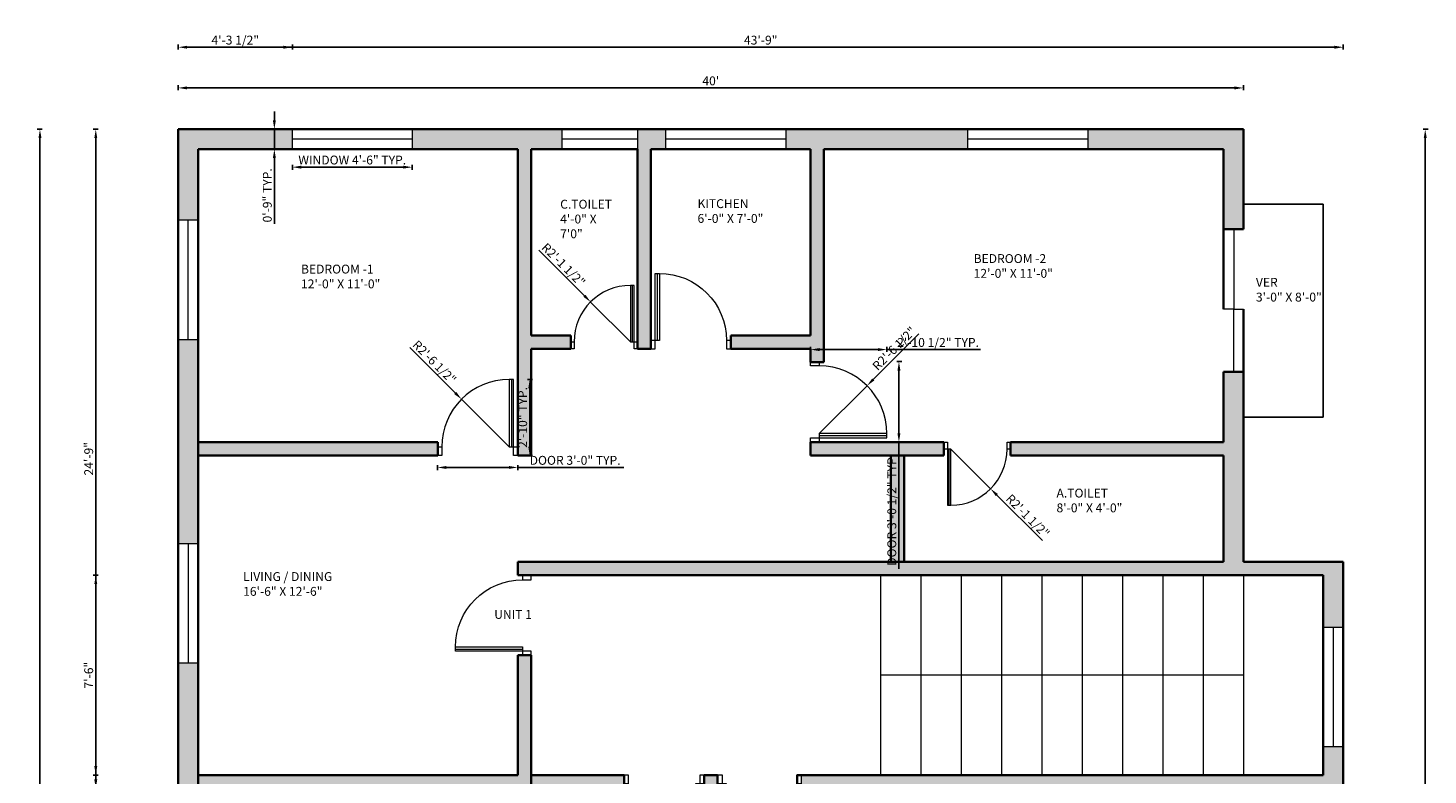
# Model space of a CAD drawing. Units: inches. Extents: x -66 to 565, y -698 to 61.
# Tile 2 of 2: x -66 to 565, y -276 to 61. Entities that reach past the tile are written whole.
import ezdxf

# ---------------------------------------------------------------- set-up
doc = ezdxf.new("R2010")
doc.units = ezdxf.units.IN
for name, color, linetype, lineweight in [('A-ANNO-DIMS', 2, 'Continuous', 18), ('A-AREA-IDEN', 7, 'Continuous', 18), ('A-DOOR', 4, 'Continuous', 18), ('A-FLOR', 7, 'Continuous', 25), ('A-FLOR-STRS', 3, 'Continuous', 18), ('A-GLAZ', 111, 'Continuous', 18), ('A-WALL', 7, 'Continuous', 35), ('A-WALL-PATT', 252, 'Continuous', 13)]:
    doc.layers.add(name, color=color, linetype=linetype, lineweight=lineweight)
doc.styles.get("Standard").update_dxf_attribs({"font": 'arial.ttf'})
doc.dimstyles.new('ISO-25', dxfattribs={"dimtxt": 4, "dimasz": 4, "dimexe": 1.25, "dimexo": 0.625, "dimtad": 1, "dimlunit": 3, "dimtxsty": 'Standard', "dimcen": 2.5, "dimadec": 0, "dimazin": 0, "dimtfac": 1, "dimtmove": 0, "dimatfit": 3, "dimfxl": 1, "dimfxlon": 1, "dimarcsym": 0})

# ---------------------------------------------------------------- blocks, each defined once
blk = doc.blocks.new('A$C296830DC')
blk.add_line((829, 853), (829, 95))
for points in [[(853, 95), (853, 853), (805, 853), (805, 95)], [(47, 95), (47, 0), (0, 0), (0, 95)], [(900, 95), (900, 0), (853, 0), (853, 95)]]:
    blk.add_lwpolyline(points, close=True)
blk.add_arc((805, 95), 758, 90, 180)
blk = doc.blocks.new('*D2')
at = {"layer": 'A-ANNO-DIMS', "color": 0, "lineweight": -2, "transparency": 16777216}
for p, q in [((1.61, 32.52), (1.61, 34.77)), ((5.61, 33.52), (477.61, 33.52)), ((481.61, 32.52), (481.61, 34.77))]:
    blk.add_line(p, q, dxfattribs=at)
at = {"layer": 'A-ANNO-DIMS', "color": 0, "transparency": 16777216}
for points in [[(5.61, 34.18), (5.61, 32.85), (1.61, 33.52)], [(477.61, 34.18), (477.61, 32.85), (481.61, 33.52)]]:
    blk.add_solid(points, dxfattribs=at)
at = {"layer": 'Defpoints', "color": 0, "transparency": 16777216}
for p in [(481.61, 33.52), (1.61, 14.91), (481.61, 14.91)]:
    blk.add_point(p, dxfattribs=at)
at = {"layer": 'A-ANNO-DIMS', "color": 0, "transparency": 16777216, "insert": (241.61, 36.18), "char_height": 4, "attachment_point": 5}
blk.add_mtext("40'", dxfattribs=at)
blk = doc.blocks.new('*D3')
at = {"layer": 'A-ANNO-DIMS', "color": 0, "lineweight": -2, "transparency": 16777216}
for p, q in [((-59.68, 14.91), (-61.93, 14.91)), ((-60.68, 10.91), (-60.68, -641.09)), ((-59.68, -645.09), (-61.93, -645.09))]:
    blk.add_line(p, q, dxfattribs=at)
at = {"layer": 'A-ANNO-DIMS', "color": 0, "transparency": 16777216}
for points in [[(-61.35, 10.91), (-60.01, 10.91), (-60.68, 14.91)], [(-61.35, -641.09), (-60.01, -641.09), (-60.68, -645.09)]]:
    blk.add_solid(points, dxfattribs=at)
at = {"layer": 'Defpoints', "color": 0, "transparency": 16777216}
for p in [(1.61, 14.91), (-60.68, -645.09), (1.61, -645.09)]:
    blk.add_point(p, dxfattribs=at)
at = {"layer": 'A-ANNO-DIMS', "color": 0, "transparency": 16777216, "insert": (-63.34, -315.09), "char_height": 4, "attachment_point": 5, "rotation": 90}
blk.add_mtext("55'", dxfattribs=at)
blk = doc.blocks.new('WIN-54IN')
blk.add_line((4.5, 54), (4.5, 0))
blk.add_lwpolyline([(0, 54), (9, 54), (9, 0), (0, 0)], close=True)
blk = doc.blocks.new('WIN-34IN')
blk.add_line((34, 4.5), (0, 4.5))
blk.add_lwpolyline([(0, 9), (34, 9), (34, 0), (0, 0)], close=True)
blk = doc.blocks.new('*D6')
at = {"layer": 'A-ANNO-DIMS', "color": 0, "lineweight": -2, "transparency": 16777216}
for p, q in [((118.49, -136.5), (118.49, -138.75)), ((122.49, -137.5), (150.61, -137.5)), ((154.61, -136.5), (154.61, -138.75)), ((154.61, -137.5), (202.36, -137.5))]:
    blk.add_line(p, q, dxfattribs=at)
at = {"layer": 'A-ANNO-DIMS', "color": 0, "transparency": 16777216}
for points in [[(122.49, -136.84), (122.49, -138.17), (118.49, -137.5)], [(150.61, -136.84), (150.61, -138.17), (154.61, -137.5)]]:
    blk.add_solid(points, dxfattribs=at)
at = {"layer": 'Defpoints', "color": 0, "transparency": 16777216}
for p in [(118.49, -132.09), (154.61, -132.09), (154.61, -137.5)]:
    blk.add_point(p, dxfattribs=at)
at = {"layer": 'A-ANNO-DIMS', "color": 0, "transparency": 16777216, "insert": (180.48, -134.81), "char_height": 4, "attachment_point": 5}
blk.add_mtext('DOOR 3\'-0" TYP.', dxfattribs=at)
blk = doc.blocks.new('*D7')
at = {"layer": 'A-ANNO-DIMS', "color": 0, "lineweight": -2, "transparency": 16777216}
for p, q in [((159.03, -97.87), (161.28, -97.87)), ((160.03, -128.09), (160.03, -101.87)), ((159.03, -132.09), (161.28, -132.09))]:
    blk.add_line(p, q, dxfattribs=at)
at = {"layer": 'A-ANNO-DIMS', "color": 0, "transparency": 16777216}
for points in [[(159.36, -101.87), (160.69, -101.87), (160.03, -97.87)], [(159.36, -128.09), (160.69, -128.09), (160.03, -132.09)]]:
    blk.add_solid(points, dxfattribs=at)
at = {"layer": 'Defpoints', "color": 0, "transparency": 16777216}
for p in [(154.61, -97.87), (160.03, -97.87), (154.61, -132.09)]:
    blk.add_point(p, dxfattribs=at)
at = {"layer": 'A-ANNO-DIMS', "color": 0, "transparency": 16777216, "insert": (157.36, -114.98), "char_height": 4, "attachment_point": 5, "rotation": 90}
blk.add_mtext('2\'-10" TYP.', dxfattribs=at)
blk = doc.blocks.new('*D10')
at = {"layer": 'A-ANNO-DIMS', "color": 0, "lineweight": -2, "transparency": 16777216}
for p, q in [((325.4, -89.83), (327.65, -89.83)), ((326.4, -93.83), (326.4, -122.09)), ((325.4, -126.09), (327.65, -126.09)), ((326.4, -126.09), (326.4, -183.16))]:
    blk.add_line(p, q, dxfattribs=at)
at = {"layer": 'A-ANNO-DIMS', "color": 0, "transparency": 16777216}
for points in [[(325.73, -93.83), (327.06, -93.83), (326.4, -89.83)], [(325.73, -122.09), (327.06, -122.09), (326.4, -126.09)]]:
    blk.add_solid(points, dxfattribs=at)
at = {"layer": 'Defpoints', "color": 0, "transparency": 16777216}
for p in [(320.96, -89.83), (320.96, -126.09), (326.4, -126.09)]:
    blk.add_point(p, dxfattribs=at)
at = {"layer": 'A-ANNO-DIMS', "color": 0, "transparency": 16777216, "insert": (323.7, -156.62), "char_height": 4, "attachment_point": 5, "rotation": 90}
blk.add_mtext('DOOR 3\'-0 1/2" TYP.', dxfattribs=at)
blk = doc.blocks.new('*D11')
at = {"layer": 'A-ANNO-DIMS', "color": 0, "lineweight": -2, "transparency": 16777216}
for p, q in [((286.61, -85.39), (286.61, -83.14)), ((290.61, -84.39), (316.96, -84.39)), ((320.96, -85.39), (320.96, -83.14)), ((320.96, -84.39), (363.09, -84.39))]:
    blk.add_line(p, q, dxfattribs=at)
at = {"layer": 'A-ANNO-DIMS', "color": 0, "transparency": 16777216}
for points in [[(290.61, -83.72), (290.61, -85.05), (286.61, -84.39)], [(316.96, -83.72), (316.96, -85.05), (320.96, -84.39)]]:
    blk.add_solid(points, dxfattribs=at)
at = {"layer": 'Defpoints', "color": 0, "transparency": 16777216}
for p in [(320.96, -84.39), (286.61, -89.83), (320.96, -89.83)]:
    blk.add_point(p, dxfattribs=at)
at = {"layer": 'A-ANNO-DIMS', "color": 0, "transparency": 16777216, "insert": (344.02, -81.69), "char_height": 4, "attachment_point": 5}
blk.add_mtext('2\'-10 1/2" TYP.', dxfattribs=at)
blk = doc.blocks.new('*D16')
at = {"layer": 'A-ANNO-DIMS', "color": 0, "lineweight": -2, "transparency": 16777216}
for p, q in [((53.05, -1.19), (53.05, -3.44)), ((57.05, -2.19), (103.05, -2.19)), ((107.05, -1.19), (107.05, -3.44))]:
    blk.add_line(p, q, dxfattribs=at)
at = {"layer": 'A-ANNO-DIMS', "color": 0, "transparency": 16777216}
for points in [[(57.05, -1.52), (57.05, -2.85), (53.05, -2.19)], [(103.05, -1.52), (103.05, -2.85), (107.05, -2.19)]]:
    blk.add_solid(points, dxfattribs=at)
at = {"layer": 'Defpoints', "color": 0, "transparency": 16777216}
for p in [(53.05, 5.91), (107.05, 5.91), (107.05, -2.19)]:
    blk.add_point(p, dxfattribs=at)
at = {"layer": 'A-ANNO-DIMS', "color": 0, "transparency": 16777216, "insert": (80.05, 0.51), "char_height": 4, "attachment_point": 5}
blk.add_mtext('WINDOW 4\'-6" TYP.', dxfattribs=at)
blk = doc.blocks.new('*D17')
at = {"layer": 'A-ANNO-DIMS', "color": 0, "lineweight": -2, "transparency": 16777216}
for p, q in [((44.95, 18.91), (44.95, 22.91)), ((45.95, 14.91), (43.7, 14.91)), ((44.95, 14.91), (44.95, 5.91)), ((45.95, 5.91), (43.7, 5.91)), ((44.95, 1.91), (44.95, -27.72))]:
    blk.add_line(p, q, dxfattribs=at)
at = {"layer": 'A-ANNO-DIMS', "color": 0, "transparency": 16777216}
for points in [[(44.29, 18.91), (45.62, 18.91), (44.95, 14.91)], [(44.29, 1.91), (45.62, 1.91), (44.95, 5.91)]]:
    blk.add_solid(points, dxfattribs=at)
at = {"layer": 'Defpoints', "color": 0, "transparency": 16777216}
for p in [(53.05, 14.91), (44.95, 5.91), (53.05, 5.91)]:
    blk.add_point(p, dxfattribs=at)
at = {"layer": 'A-ANNO-DIMS', "color": 0, "transparency": 16777216, "insert": (42.29, -14.9), "char_height": 4, "attachment_point": 5, "rotation": 90}
blk.add_mtext('0\'-9" TYP.', dxfattribs=at)
blk = doc.blocks.new('*D20')
at = {"layer": 'A-ANNO-DIMS', "color": 0, "lineweight": -2, "transparency": 16777216}
for p, q in [((1.61, 50.86), (1.61, 53.11)), ((5.61, 51.86), (522.61, 51.86)), ((526.61, 50.86), (526.61, 53.11))]:
    blk.add_line(p, q, dxfattribs=at)
at = {"layer": 'A-ANNO-DIMS', "color": 0, "transparency": 16777216}
for points in [[(5.61, 52.53), (5.61, 51.2), (1.61, 51.86)], [(522.61, 52.53), (522.61, 51.2), (526.61, 51.86)]]:
    blk.add_solid(points, dxfattribs=at)
at = {"layer": 'Defpoints', "color": 0, "transparency": 16777216}
for p in [(526.61, 51.86), (1.61, 14.91), (526.61, -180.09)]:
    blk.add_point(p, dxfattribs=at)
at = {"layer": 'A-ANNO-DIMS', "color": 0, "transparency": 16777216, "insert": (264.11, 54.53), "char_height": 4, "attachment_point": 5}
blk.add_mtext('43\'-9"', dxfattribs=at)
blk = doc.blocks.new('*D21')
at = {"layer": 'A-ANNO-DIMS', "color": 0, "lineweight": -2, "transparency": 16777216}
for p, q in [((562.56, 14.91), (564.81, 14.91)), ((563.56, 10.91), (563.56, -641.09)), ((562.56, -645.09), (564.81, -645.09))]:
    blk.add_line(p, q, dxfattribs=at)
at = {"layer": 'A-ANNO-DIMS', "color": 0, "transparency": 16777216}
for points in [[(562.89, 10.91), (564.23, 10.91), (563.56, 14.91)], [(562.89, -641.09), (564.23, -641.09), (563.56, -645.09)]]:
    blk.add_solid(points, dxfattribs=at)
at = {"layer": 'Defpoints', "color": 0, "transparency": 16777216}
for p in [(481.61, 14.91), (526.61, -645.09), (563.56, -645.09)]:
    blk.add_point(p, dxfattribs=at)
at = {"layer": 'A-ANNO-DIMS', "color": 0, "transparency": 16777216, "insert": (560.89, -315.09), "char_height": 4, "attachment_point": 5, "rotation": 90}
blk.add_mtext('55\'-0"', dxfattribs=at)
blk = doc.blocks.new('*D22')
at = {"layer": 'A-ANNO-DIMS', "color": 0, "lineweight": -2, "transparency": 16777216}
for p, q in [((-34.52, 14.91), (-36.77, 14.91)), ((-35.52, 10.91), (-35.52, -278.09)), ((-34.52, -282.09), (-36.77, -282.09))]:
    blk.add_line(p, q, dxfattribs=at)
at = {"layer": 'A-ANNO-DIMS', "color": 0, "transparency": 16777216}
for points in [[(-36.19, 10.91), (-34.86, 10.91), (-35.52, 14.91)], [(-36.19, -278.09), (-34.86, -278.09), (-35.52, -282.09)]]:
    blk.add_solid(points, dxfattribs=at)
at = {"layer": 'Defpoints', "color": 0, "transparency": 16777216}
for p in [(1.61, 14.91), (-35.52, -282.09), (10.61, -282.09)]:
    blk.add_point(p, dxfattribs=at)
at = {"layer": 'A-ANNO-DIMS', "color": 0, "transparency": 16777216, "insert": (-38.19, -133.59), "char_height": 4, "attachment_point": 5, "rotation": 90}
blk.add_mtext('24\'-9"', dxfattribs=at)
blk = doc.blocks.new('*D24')
at = {"layer": 'A-ANNO-DIMS', "color": 0, "lineweight": -2, "transparency": 16777216}
for p, q in [((-34.52, -186.09), (-36.77, -186.09)), ((-35.52, -190.09), (-35.52, -272.09)), ((-34.52, -276.09), (-36.77, -276.09))]:
    blk.add_line(p, q, dxfattribs=at)
at = {"layer": 'A-ANNO-DIMS', "color": 0, "transparency": 16777216}
for points in [[(-36.19, -190.09), (-34.86, -190.09), (-35.52, -186.09)], [(-36.19, -272.09), (-34.86, -272.09), (-35.52, -276.09)]]:
    blk.add_solid(points, dxfattribs=at)
at = {"layer": 'Defpoints', "color": 0, "transparency": 16777216}
for p in [(318.11, -186.09), (-35.52, -276.09), (318.11, -276.09)]:
    blk.add_point(p, dxfattribs=at)
at = {"layer": 'A-ANNO-DIMS', "color": 0, "transparency": 16777216, "insert": (-38.19, -231.09), "char_height": 4, "attachment_point": 5, "rotation": 90}
blk.add_mtext('7\'-6"', dxfattribs=at)
blk = doc.blocks.new('*D27')
at = {"layer": 'A-ANNO-DIMS', "color": 0, "lineweight": -2, "transparency": 16777216}
for p, q in [((1.61, 50.86), (1.61, 53.11)), ((5.61, 51.86), (49.05, 51.86)), ((53.05, 50.86), (53.05, 53.11))]:
    blk.add_line(p, q, dxfattribs=at)
at = {"layer": 'A-ANNO-DIMS', "color": 0, "transparency": 16777216}
for points in [[(5.61, 52.53), (5.61, 51.2), (1.61, 51.86)], [(49.05, 52.53), (49.05, 51.2), (53.05, 51.86)]]:
    blk.add_solid(points, dxfattribs=at)
at = {"layer": 'Defpoints', "color": 0, "transparency": 16777216}
for p in [(53.05, 51.86), (1.61, 14.91), (53.05, 14.91)]:
    blk.add_point(p, dxfattribs=at)
at = {"layer": 'A-ANNO-DIMS', "color": 0, "transparency": 16777216, "insert": (27.33, 54.56), "char_height": 4, "attachment_point": 5}
blk.add_mtext('4\'-3 1/2"', dxfattribs=at)
blk = doc.blocks.new('*D31')
at = {"layer": 'A-ANNO-DIMS', "color": 0, "lineweight": -2, "transparency": 16777216}
for p, q in [((335.37, -77.32), (314.84, -97.85)), ((290.43, -122.27), (312.02, -100.68))]:
    blk.add_line(p, q, dxfattribs=at)
at = {"layer": 'A-ANNO-DIMS', "color": 0, "transparency": 16777216}
blk.add_solid([(314.37, -97.38), (315.32, -98.32), (312.02, -100.68)], dxfattribs=at)
at = {"layer": 'Defpoints', "color": 0, "transparency": 16777216}
for p in [(312.02, -100.68), (290.43, -122.27)]:
    blk.add_point(p, dxfattribs=at)
at = {"layer": 'A-ANNO-DIMS', "color": 0, "transparency": 16777216, "insert": (324.62, -84.27), "char_height": 4, "attachment_point": 5, "rotation": 45.00056}
blk.add_mtext('R2\'-6 1/2"', dxfattribs=at)
blk = doc.blocks.new('*D32')
at = {"layer": 'A-ANNO-DIMS', "color": 0, "lineweight": -2, "transparency": 16777216}
for p, q in [((105.94, -83.42), (126.47, -103.95)), ((150.81, -128.28), (129.3, -106.78))]:
    blk.add_line(p, q, dxfattribs=at)
at = {"layer": 'A-ANNO-DIMS', "color": 0, "transparency": 16777216}
blk.add_solid([(126.94, -103.48), (126, -104.42), (129.3, -106.78)], dxfattribs=at)
at = {"layer": 'Defpoints', "color": 0, "transparency": 16777216}
for p in [(129.3, -106.78), (150.81, -128.28)]:
    blk.add_point(p, dxfattribs=at)
at = {"layer": 'A-ANNO-DIMS', "color": 0, "transparency": 16777216, "insert": (116.7, -90.37), "char_height": 4, "attachment_point": 5, "rotation": 315.00004}
blk.add_mtext('R2\'-6 1/2"', dxfattribs=at)
blk = doc.blocks.new('*D34')
at = {"layer": 'A-ANNO-DIMS', "color": 0, "lineweight": -2, "transparency": 16777216}
for p, q in [((164.11, -39.59), (184.64, -60.12)), ((205.43, -80.91), (187.47, -62.95))]:
    blk.add_line(p, q, dxfattribs=at)
at = {"layer": 'A-ANNO-DIMS', "color": 0, "transparency": 16777216}
blk.add_solid([(185.11, -59.65), (184.17, -60.59), (187.47, -62.95)], dxfattribs=at)
at = {"layer": 'Defpoints', "color": 0, "transparency": 16777216}
for p in [(187.47, -62.95), (205.43, -80.91)]:
    blk.add_point(p, dxfattribs=at)
at = {"layer": 'A-ANNO-DIMS', "color": 0, "transparency": 16777216, "insert": (174.87, -46.54), "char_height": 4, "attachment_point": 5, "rotation": 315.00004}
blk.add_mtext('R2\'-1 1/2"', dxfattribs=at)
blk = doc.blocks.new('*D35')
at = {"layer": 'A-ANNO-DIMS', "color": 0, "lineweight": -2, "transparency": 16777216}
for p, q in [((349.83, -129.24), (367.7, -147.11)), ((391.06, -170.47), (370.53, -149.94))]:
    blk.add_line(p, q, dxfattribs=at)
at = {"layer": 'A-ANNO-DIMS', "color": 0, "transparency": 16777216}
blk.add_solid([(371, -149.47), (370.05, -150.41), (367.7, -147.11)], dxfattribs=at)
at = {"layer": 'Defpoints', "color": 0, "transparency": 16777216}
for p in [(349.83, -129.24), (367.7, -147.11)]:
    blk.add_point(p, dxfattribs=at)
at = {"layer": 'A-ANNO-DIMS', "color": 0, "transparency": 16777216, "insert": (384.11, -159.72), "char_height": 4, "attachment_point": 5, "rotation": 315.00072}
blk.add_mtext('R2\'-1 1/2"', dxfattribs=at)

msp = doc.modelspace()

# ---------------------------------------------------------------- hatches: boundary and pattern name
at = {"layer": 'A-WALL-PATT'}
h = msp.add_hatch(color=256, dxfattribs=at)
h.dxf.hatch_style = 1
h.paths.add_polyline_path([(53.054, 14.914), (1.609, 14.914), (1.609, -25.926), (10.609, -25.926), (10.609, 5.914), (53.054, 5.914)])
h.paths.add_polyline_path([(174.609, 14.914), (107.054, 14.914), (107.054, 5.914), (154.609, 5.914), (154.609, -132.086), (160.609, -132.086), (160.609, -84.086), (178.441, -84.086), (178.441, -80.91), (178.609, -78.086), (160.609, -78.086), (160.609, 5.914), (174.609, 5.914)])
h.paths.add_polyline_path([(357.494, 14.914), (275.363, 14.914), (275.363, 5.914), (286.609, 5.914), (286.609, -78.086), (250.609, -78.086), (250.609, -84.086), (286.609, -84.086), (286.609, -89.827), (290.425, -89.827), (290.425, -90.086), (292.609, -90.086), (292.609, 5.914), (357.494, 5.914)])
h.paths.add_polyline_path([(221.363, 14.914), (208.609, 14.914), (208.609, 5.914), (208.609, -84.086), (214.609, -84.086), (214.609, 5.914), (221.363, 5.914)])
h.paths.add_polyline_path([(481.609, 14.914), (411.494, 14.914), (411.494, 5.914), (472.609, 5.914), (472.609, -30.057), (477.316, -30.057), (481.609, -30.057)])
h.paths.add_polyline_path([(481.609, -94.45), (472.609, -94.45), (472.609, -126.086), (376.678, -126.086), (376.678, -129.244), (376.609, -132.086), (472.609, -132.086), (472.609, -180.086), (154.609, -180.086), (154.609, -186.086), (481.609, -186.086), (517.609, -186.086), (517.609, -209.408), (526.609, -209.408), (526.609, -180.086), (523.609, -180.086), (481.609, -180.086)])
h.paths.add_polyline_path([(346.609, -126.086), (292.609, -126.086), (286.609, -126.086), (286.609, -132.086), (292.609, -132.086), (346.609, -132.086)], flags=17)
h.paths.add_polyline_path([(118.491, -128.284), (118.609, -126.086), (10.609, -126.086), (10.609, -132.086), (118.491, -132.086)])
h.paths.add_polyline_path([(10.609, -79.926), (1.609, -79.926), (1.609, -171.746), (10.609, -171.746)])
h.paths.add_polyline_path([(10.609, -225.746), (1.609, -225.746), (1.609, -303.953), (10.609, -303.953)])
h.paths.add_polyline_path([(160.609, -222.168), (156.831, -222.168), (154.609, -222.086), (154.609, -276.086), (10.609, -276.086), (10.609, -282.086), (136.609, -282.086), (136.609, -408.086), (142.609, -408.086), (142.609, -282.086), (160.609, -282.086)])
h.paths.add_polyline_path([(202.609, -276.086), (160.609, -276.086), (160.609, -282.086), (202.609, -282.086)])
h.paths.add_polyline_path([(526.609, -263.408), (517.609, -263.408), (517.609, -276.086), (282.342, -276.086), (282.342, -280.017), (280.606, -280.017), (280.606, -282.086), (340.609, -282.086), (340.609, -408.086), (346.609, -408.086), (346.609, -404.294), (346.609, -282.086), (517.609, -282.086), (517.609, -323.855), (526.609, -323.855), (526.609, -282.086)])
h.paths.add_polyline_path([(244.609, -276.086), (238.609, -276.086), (238.609, -279.866), (238.609, -522.086), (244.609, -522.086)])
h.paths.add_polyline_path([(526.609, -377.855), (517.609, -377.855), (517.609, -425.984), (526.609, -425.984)])
h.paths.add_polyline_path([(517.609, -402.086), (382.609, -402.086), (382.609, -404.294), (382.631, -404.294), (382.631, -408.086), (433.609, -408.086), (433.609, -432.07), (436.561, -432.07), (439.609, -432.086), (439.609, -408.086), (517.609, -408.086)])
h.paths.add_polyline_path([(517.609, -462.086), (439.609, -462.086), (340.609, -462.086), (340.609, -468.086), (344.391, -468.086), (439.609, -468.086), (517.609, -468.086)])
h.paths.add_polyline_path([(526.609, -459.984), (517.609, -459.984), (517.609, -500.965), (526.609, -500.965)])
h.paths.add_polyline_path([(526.609, -554.965), (517.609, -554.965), (517.609, -594.086), (526.609, -594.086)])
h.paths.add_polyline_path([(436.609, -588.086), (426.99, -588.086), (426.99, -592.769), (426.99, -636.086), (380.508, -636.086), (380.508, -645.086), (436.609, -645.086)])
h.paths.add_polyline_path([(346.609, -504.086), (340.609, -504.086), (340.609, -522.086), (282.342, -522.086), (282.342, -526.045), (282.342, -528.086), (340.609, -528.086), (340.609, -624.086), (319.481, -624.086), (319.481, -633.086), (346.609, -633.086), (346.609, -594.086), (382.609, -594.086), (382.609, -592.769), (382.497, -592.769), (382.497, -588.086), (346.609, -588.086)])
h.paths.add_polyline_path([(265.481, -624.086), (244.609, -624.086), (244.609, -522.086), (238.609, -522.086), (238.609, -624.086), (209.858, -624.086), (209.858, -633.086), (265.481, -633.086)])
h.paths.add_polyline_path([(142.609, -528.086), (202.609, -528.086), (202.609, -522.086), (142.609, -522.086), (142.609, -504.167), (138.764, -504.167), (136.609, -504.086), (136.609, -588.086), (100.609, -588.086), (100.609, -594.086), (136.609, -594.086), (136.609, -636.086), (136.6, -636.086), (136.6, -645.086), (142.609, -645.086), (142.609, -633.086), (155.858, -633.086), (155.858, -624.086), (142.609, -624.086), (142.609, -588.086)])
h.paths.add_polyline_path([(102.6, -636.086), (70.609, -636.086), (70.609, -588.086), (64.609, -588.086), (64.609, -645.086), (70.609, -645.086), (102.6, -645.086)])
h.paths.add_polyline_path([(10.609, -551.068), (1.609, -551.068), (1.609, -594.086), (10.609, -594.086)])
h.paths.add_polyline_path([(10.609, -468.086), (88.609, -468.086), (138.764, -468.086), (138.764, -467.878), (142.609, -467.878), (142.609, -462.086), (94.536, -462.086), (94.536, -462.142), (91.375, -462.142), (88.609, -462.086), (10.609, -462.086), (10.609, -459.984), (1.609, -459.984), (1.609, -497.068), (10.609, -497.068)])
h.paths.add_polyline_path([(100.609, -402.086), (10.609, -402.086), (10.609, -357.953), (1.609, -357.953), (1.609, -425.984), (10.609, -425.984), (10.609, -408.086), (88.609, -408.086), (88.609, -432.086), (94.609, -432.086), (94.609, -408.086), (100.609, -408.086)])
h = msp.add_hatch(color=256, dxfattribs=at)
h.dxf.hatch_style = 1
h.paths.add_polyline_path([(328.76, -132.086), (322.76, -132.086), (322.76, -180.086), (328.76, -180.086)])

# ---------------------------------------------------------------- linework, layer by layer
at = {"layer": 'A-DOOR'}
msp.add_lwpolyline([(472.609, -30.057), (477.316, -30.057), (477.316, -66.181), (472.609, -66.181)], close=True, dxfattribs=at)
msp.add_lwpolyline([(477.316, -94.45), (477.316, -66.222), (481.609, -66.222)], dxfattribs=at)
at = {"layer": 'A-FLOR'}
for p, q in [((481.609, -18.873), (517.609, -18.873)), ((517.609, -18.873), (517.609, -114.873)), ((517.609, -114.873), (481.609, -114.873))]:
    msp.add_line(p, q, dxfattribs=at)
at = {"layer": 'A-FLOR-STRS'}
for p, q in [((318.109, -186.086), (318.109, -276.086)), ((336.275, -186.086), (336.275, -276.086)), ((354.442, -186.086), (354.442, -276.086)), ((372.609, -186.086), (372.609, -276.086)), ((390.775, -186.086), (390.775, -276.086)), ((408.942, -186.086), (408.942, -276.086)), ((427.109, -186.086), (427.109, -276.086)), ((445.275, -186.086), (445.275, -276.086)), ((463.442, -186.086), (463.442, -276.086)), ((481.609, -186.086), (481.609, -276.086)), ((481.609, -186.086), (481.609, -276.086)), ((481.609, -231.086), (318.109, -231.086))]:
    msp.add_line(p, q, dxfattribs=at)
at = {"layer": 'A-WALL'}
for p, q in [((1.609, 14.914), (481.609, 14.914)), ((1.609, -645.086), (1.609, 14.914)), ((481.609, 14.914), (481.609, -30.057)), ((10.609, 5.914), (154.609, 5.914)), ((10.609, -402.086), (10.609, 5.914)), ((154.609, -132.086), (154.609, 5.914)), ((160.609, 5.914), (208.609, 5.914)), ((160.609, -78.086), (160.609, 5.914)), ((208.609, -84.086), (208.609, 5.914)), ((214.609, 5.914), (286.609, 5.914)), ((214.609, -84.086), (214.609, 5.914)), ((286.609, -78.086), (286.609, 5.914)), ((292.609, 5.914), (472.609, 5.914)), ((292.609, -90.086), (292.609, 5.914)), ((472.609, 5.914), (472.609, -66.181)), ((481.609, -30.057), (472.609, -30.057)), ((481.609, -66.222), (481.609, -180.086)), ((160.609, -78.086), (178.609, -78.086)), ((178.609, -78.086), (178.609, -84.086)), ((250.609, -78.086), (286.609, -78.086)), ((250.609, -84.086), (250.609, -78.086)), ((160.609, -84.086), (178.609, -84.086)), ((160.609, -132.086), (160.609, -84.086)), ((214.609, -84.086), (208.609, -84.086)), ((250.609, -84.086), (286.609, -84.086)), ((286.609, -90.086), (286.609, -84.086)), ((292.609, -90.086), (286.609, -90.086)), ((472.609, -94.45), (481.609, -94.45)), ((472.609, -94.45), (472.609, -126.086)), ((10.609, -126.086), (118.609, -126.086)), ((118.609, -126.086), (118.609, -132.086)), ((292.609, -126.086), (286.609, -126.086)), ((286.609, -132.086), (286.609, -126.086)), ((292.609, -126.086), (346.609, -126.086)), ((346.609, -132.086), (346.609, -126.086)), ((376.609, -132.086), (376.609, -126.086)), ((376.609, -126.086), (472.609, -126.086)), ((10.609, -132.086), (118.609, -132.086)), ((154.609, -132.086), (160.609, -132.086)), ((292.609, -132.086), (286.609, -132.086)), ((292.609, -132.086), (346.609, -132.086)), ((322.76, -180.086), (322.76, -132.086)), ((328.76, -180.086), (328.76, -132.086)), ((376.609, -132.086), (472.609, -132.086)), ((472.609, -132.086), (472.609, -180.086)), ((154.609, -180.086), (472.609, -180.086)), ((154.609, -186.086), (154.609, -180.086)), ((481.609, -180.086), (523.609, -180.086)), ((523.609, -180.086), (526.609, -180.086)), ((526.609, -180.086), (526.609, -282.086)), ((154.609, -186.086), (481.609, -186.086)), ((481.609, -186.086), (517.609, -186.086)), ((517.609, -186.086), (517.609, -276.086)), ((154.609, -276.086), (154.609, -222.086)), ((160.609, -222.086), (154.609, -222.086)), ((160.609, -221.785), (160.609, -221.785)), ((160.609, -282.086), (160.609, -222.086)), ((154.609, -276.086), (10.609, -276.086)), ((202.609, -276.086), (160.609, -276.086)), ((202.609, -282.086), (202.609, -276.086)), ((238.609, -276.086), (238.609, -624.086)), ((244.609, -276.086), (238.609, -276.086)), ((244.609, -276.086), (244.609, -624.086)), ((517.609, -276.086), (280.606, -276.086)), ((280.606, -282.086), (280.606, -276.086))]:
    msp.add_line(p, q, dxfattribs=at)

# ---------------------------------------------------------------- block references
at = {"layer": 'A-DOOR'}
for p, xscale, yscale, zscale in [((250.583, -84.102), -0.0399314266132186, 0.0399314266132186, 0.0399314266132186), ((178.441, -84.086), 0.0335195759141932, 0.0335195759141932, 0.0335195759141932), ((118.491, -132.086), 0.040130878893069, 0.040130878893069, 0.040130878893069)]:
    msp.add_blockref('A$C296830DC', p, dxfattribs=dict(at, xscale=xscale, yscale=yscale, zscale=zscale))
for p, xscale, yscale, zscale, rotation in [((286.609, -89.827), 0.040287546519816, 0.040287546519816, 0.040287546519816, 270), ((376.678, -126.086), 0.0333423284861908, 0.0333423284861908, 0.0333423284861908, 180), ((160.609, -186.28), -0.0398750419985196, 0.0398750419985196, 0.0398750419985196, 90), ((202.697, -276.086), -0.0399020096887821, 0.0399020096887821, 0.0399020096887821, 180), ((282.342, -276.058), 0.0417895516625183, 0.0417895516625183, 0.0417895516625183, 180)]:
    msp.add_blockref('A$C296830DC', p, dxfattribs=dict(at, xscale=xscale, yscale=yscale, zscale=zscale, rotation=rotation))
at = {"layer": 'A-GLAZ', "rotation": 270.0000000000001}
for p in [(53.054, 14.914), (221.363, 14.914), (357.494, 14.914)]:
    msp.add_blockref('WIN-54IN', p, dxfattribs=at)
at = {"layer": 'A-GLAZ'}
for name, p in [('WIN-34IN', (174.609, 5.914)), ('WIN-54IN', (1.428, -79.926)), ('WIN-54IN', (1.616, -225.747)), ('WIN-54IN', (517.597, -263.408))]:
    msp.add_blockref(name, p, dxfattribs=at)

# ---------------------------------------------------------------- texts
at = {"layer": 'A-AREA-IDEN', "char_height": 4, "attachment_point": 1}
for s, width, insert in [('C.TOILET\\P4\'-0" X 7\'0"', 27.53191, (173.748, -16.883)), ('KITCHEN\\P6\'-0" X 7\'-0"', 33.56271, (235.63, -16.621)), ('BEDROOM -2\\P12\'-0" X 11\'-0"', 85.65337, (360.055, -41.378)), ('BEDROOM -1\\P12\'-0" X 11\'-0"', 75.98686, (56.959, -46.115)), ('VER\\P3\'-0" X 8\'-0"', 33.48682, (487.26, -52.074)), ('A.TOILET\\P8\'-0" X 4\'-0"', 44.97756, (397.41, -147.048)), ('LIVING / DINING\\P16\'-6" X 12\'-6"', 64.84212, (30.884, -184.669)), ('UNIT 1', 31.79191, (144.024, -201.717))]:
    msp.add_mtext_dynamic_manual_height_columns(s, width=width, gutter_width=12.5, heights=[0], dxfattribs=dict(at, insert=insert))

# ---------------------------------------------------------------- dimensions: what is measured, and where the dimension line sits
at = {"layer": 'A-ANNO-DIMS'}
for base, p2, override, picture, middle in [((53.054, 51.864), (53.054, 14.914), {"dimdec": 1, "dimlfac": 1, "dimrnd": 0, "dimzin": 1, "dimdsep": 46, "dimlunit": 4, "dimfrac": 2}, '*D27', (27.331, 54.559)), ((526.609, 51.864), (526.609, -180.086), {"dimdec": 1, "dimlfac": 1, "dimrnd": 0, "dimzin": 1, "dimdsep": 46, "dimlunit": 4, "dimfrac": 2}, '*D20', (264.109, 54.533)), ((481.609, 33.516), (481.609, 14.914), {"dimclrd": 0, "dimclre": 0, "dimclrt": 0}, '*D2', (241.609, 36.184))]:
    dim = msp.add_linear_dim(base=base, p1=(1.609, 14.914), p2=p2, dimstyle='ISO-25', override=override, dxfattribs=at)
    dim.commit()
    dim.dimension.update_dxf_attribs({"geometry": picture, "text_midpoint": middle})
for base, p1, p2, angle, text, picture, middle in [((44.954, 5.914), (53.054, 14.914), (53.054, 5.914), 270, '<> TYP.', '*D17', (42.287, -14.902)), ((107.054, -2.186), (53.054, 5.914), (107.054, 5.914), 0, 'WINDOW <> TYP.', '*D16', (80.054, 0.509)), ((326.398, -126.086), (320.959, -89.827), (320.959, -126.086), 270, 'DOOR <> TYP.', '*D10', (323.702, -156.621)), ((160.026, -97.869), (154.609, -132.086), (154.609, -97.869), 90, '<> TYP.', '*D7', (157.359, -114.977))]:
    dim = msp.add_linear_dim(base=base, p1=p1, p2=p2, angle=angle, text=text, dimstyle='ISO-25', override={"dimdec": 1, "dimlfac": 1, "dimrnd": 0, "dimzin": 1, "dimdsep": 46, "dimlunit": 4, "dimfrac": 2}, dxfattribs=at)
    dim.commit()
    dim.dimension.update_dxf_attribs({"geometry": picture, "text_midpoint": middle})
for base, p1, p2, override, picture, middle in [((-60.681, -645.086), (1.609, 14.914), (1.609, -645.086), {"dimclrd": 0, "dimclre": 0, "dimclrt": 0}, '*D3', (-63.34, -315.086)), ((-35.523, -282.086), (1.609, 14.914), (10.609, -282.086), {"dimdec": 1, "dimlfac": 1, "dimrnd": 0, "dimzin": 1, "dimdsep": 46, "dimlunit": 4, "dimfrac": 2}, '*D22', (-38.19, -133.586)), ((563.559, -645.086), (481.609, 14.914), (526.609, -645.086), {"dimdec": 1, "dimlfac": 1, "dimrnd": 0, "dimzin": 1, "dimdsep": 46, "dimlunit": 4, "dimfrac": 2}, '*D21', (560.891, -315.086)), ((-35.523, -276.086), (318.109, -186.086), (318.109, -276.086), {"dimdec": 1, "dimlfac": 1, "dimrnd": 0, "dimzin": 1, "dimdsep": 46, "dimlunit": 4, "dimfrac": 2}, '*D24', (-38.19, -231.086))]:
    dim = msp.add_linear_dim(base=base, p1=p1, p2=p2, angle=90, dimstyle='ISO-25', override=override, dxfattribs=at)
    dim.commit()
    dim.dimension.update_dxf_attribs({"geometry": picture, "text_midpoint": middle})
for center, mpoint, picture, middle in [((205.433, -80.91), (187.47, -62.947), '*D34', (174.867, -46.535)), ((290.425, -122.269), (312.016, -100.678), '*D31', (324.618, -84.267)), ((150.807, -128.284), (129.3, -106.777), '*D32', (116.698, -90.366)), ((349.829, -129.244), (367.698, -147.113), '*D35', (384.109, -159.715))]:
    dim = msp.add_radius_dim(center=center, mpoint=mpoint, dimstyle='ISO-25', override={"dimdec": 1, "dimlfac": 1, "dimrnd": 0, "dimzin": 1, "dimdsep": 46, "dimlunit": 4, "dimfrac": 2}, dxfattribs=at)
    dim.commit()
    dim.dimension.update_dxf_attribs({"geometry": picture, "text_midpoint": middle})
for base, p1, p2, text, picture, middle in [((320.9592, -84.3881), (286.6087, -89.8269), (320.9592, -89.8269), '<> TYP.', '*D11', (344.0235, -81.6949)), ((154.609, -137.503), (118.491, -132.086), (154.609, -132.086), 'DOOR <> TYP.', '*D6', (180.483, -134.807))]:
    dim = msp.add_linear_dim(base=base, p1=p1, p2=p2, text=text, dimstyle='ISO-25', override={"dimdec": 1, "dimlfac": 1, "dimrnd": 0, "dimzin": 1, "dimdsep": 46, "dimlunit": 4, "dimfrac": 2}, dxfattribs=at)
    dim.commit()
    dim.dimension.update_dxf_attribs({"geometry": picture, "text_midpoint": middle})

doc.saveas('drawing.dxf')
